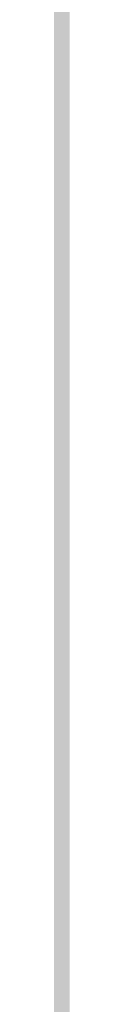
# Model space of a CAD drawing. Units: inches. Extents: x 2083 to 3317, y 1141 to 2115.
# Tile 200 of 256: x 3126.9558 to 3126.9579, y 1263.6134 to 1264.1307. Entities that reach past the tile are written whole.
import ezdxf

# ---------------------------------------------------------------- set-up
doc = ezdxf.new("R2010")
doc.units = ezdxf.units.IN
doc.layers.add('A-ANNO-DIMS', color=2, linetype='Continuous', lineweight=18)
doc.layers.add('A-WALL-PATT', color=251, linetype='Continuous', lineweight=13, true_color=0x636466)
doc.styles.get("Standard").update_dxf_attribs({"font": 'arial.ttf'})
doc.dimstyles.new('ISO-25', dxfattribs={"dimtxt": 12, "dimasz": 12, "dimexe": 1.25, "dimexo": 0.625, "dimtad": 1, "dimlunit": 3, "dimtxsty": 'Standard', "dimcen": 2.5, "dimadec": 0, "dimazin": 0, "dimtfac": 1, "dimtmove": 0, "dimatfit": 3, "dimfxl": 1, "dimarcsym": 0})

# ---------------------------------------------------------------- blocks, each defined once
blk = doc.blocks.new('*D26')
at = {"layer": 'A-ANNO-DIMS', "color": 0, "lineweight": -2, "transparency": 16777216}
for p, q in [((3088.98584, 1274.91509), (3088.98584, 1270.95196)), ((3111.24004, 1274.91509), (3111.24004, 1270.95196)), ((3076.98584, 1272.20196), (2840.26245, 1272.20196)), ((3111.24004, 1272.20196), (3088.98584, 1272.20196)), ((3123.24004, 1272.20196), (3135.24004, 1272.20196))]:
    blk.add_line(p, q, dxfattribs=at)
at = {"layer": 'A-ANNO-DIMS', "color": 0, "transparency": 16777216}
for points in [[(3076.98584, 1274.20196), (3076.98584, 1270.20196), (3088.98584, 1272.20196)], [(3123.24004, 1274.20196), (3123.24004, 1270.20196), (3111.24004, 1272.20196)]]:
    blk.add_solid(points, dxfattribs=at)
at = {"layer": 'Defpoints', "color": 0, "transparency": 16777216}
for p in [(3088.98584, 1275.54009), (3111.24004, 1275.54009), (3088.98584, 1272.20196)]:
    blk.add_point(p, dxfattribs=at)
at = {"layer": 'A-ANNO-DIMS', "color": 0, "transparency": 16777216, "insert": (2952.62415, 1279.0316), "char_height": 12, "attachment_point": 5}
blk.add_mtext('NIGHTSTAND 1\'-10 1/2" TYP.', dxfattribs=at)
blk = doc.blocks.new('*D27')
at = {"layer": 'A-ANNO-DIMS', "color": 0, "lineweight": -2, "transparency": 16777216}
for p, q in [((3114.57817, 1309.79428), (3114.57817, 1321.79428)), ((3111.86504, 1297.79428), (3115.82817, 1297.79428)), ((3114.57817, 1297.79428), (3114.57817, 1275.54009)), ((3111.86504, 1275.54009), (3115.82817, 1275.54009)), ((3114.57817, 1263.54009), (3114.57817, 1140.98859))]:
    blk.add_line(p, q, dxfattribs=at)
at = {"layer": 'A-ANNO-DIMS', "color": 0, "transparency": 16777216}
for points in [[(3112.57817, 1309.79428), (3116.57817, 1309.79428), (3114.57817, 1297.79428)], [(3112.57817, 1263.54009), (3116.57817, 1263.54009), (3114.57817, 1275.54009)]]:
    blk.add_solid(points, dxfattribs=at)
at = {"layer": 'Defpoints', "color": 0, "transparency": 16777216}
for p in [(3111.24004, 1297.79428), (3111.24004, 1275.54009), (3114.57817, 1275.54009)]:
    blk.add_point(p, dxfattribs=at)
at = {"layer": 'A-ANNO-DIMS', "color": 0, "transparency": 16777216, "insert": (3107.74853, 1196.26434), "char_height": 12, "attachment_point": 5, "rotation": 90}
blk.add_mtext('1\'-10 1/2" TYP.', dxfattribs=at)

msp = doc.modelspace()

# ---------------------------------------------------------------- hatches: boundary and pattern name
at = {"layer": 'A-WALL-PATT'}
h = msp.add_hatch(color=256, dxfattribs=at)
h.dxf.hatch_style = 1
h.paths.add_polyline_path([(3126.95978, 2020.76136), (2748.95978, 2020.76136), (2604.95978, 2020.76136), (2226.95978, 2020.76136), (2226.95978, 1702.76136), (2466.95978, 1702.76136), (2466.95978, 1582.76136), (2418.95978, 1582.76136), (2418.95978, 1477.76136), (2226.95978, 1477.76136), (2226.95978, 1263.26136), (2544.95978, 1263.26136), (2544.95978, 1411.76136), (2604.95978, 1411.76136), (2685.95978, 1411.76136), (2685.95978, 1420.76136), (2604.95978, 1420.76136), (2604.95978, 1573.76136), (2604.95978, 1702.76136), (2604.95978, 2011.76136), (2748.95978, 2011.76136), (2748.95978, 1702.76136), (2862.95978, 1702.76136), (2862.95978, 1621.76136), (2871.95978, 1621.76136), (2871.95978, 1702.76136), (2883.95978, 1702.76136), (2883.95978, 1706.93946, -0.026459), (2883.95978, 1711.76136), (2757.95978, 1711.76136), (2757.95978, 1807.76136), (2787.95978, 1807.76136), (2787.95978, 1812.26136), (2757.95978, 1812.26136), (2757.95978, 2011.76136), (2877.95978, 2011.76136), (2877.95978, 1812.26136), (2847.95978, 1812.26136), (2847.95978, 1807.76136), (2889.83574, 1807.76136), (2889.83574, 1812.26136), (2882.45978, 1812.26136), (2882.45978, 2011.76136), (3117.95978, 2011.76136), (3117.95978, 1812.26136), (2937.83574, 1812.26136), (2937.83574, 1807.76136), (2995.70978, 1807.76136), (2995.70978, 1796.11767), (3000.20978, 1796.11767), (3000.20978, 1807.76136), (3117.95978, 1807.76136), (3117.95978, 1711.76136), (3000.20978, 1711.76136), (3000.20978, 1760.11767), (2998.5727, 1760.11767, -0.020711), (2995.70978, 1760.11767), (2995.70978, 1711.76136), (2931.95978, 1711.76136), (2931.95978, 1702.76136), (3126.95978, 1702.76136)])
h.paths.add_polyline_path([(2471.45978, 2011.76136), (2471.45978, 1810.01136), (2462.71694, 1810.01136), (2462.71694, 1805.51136), (2505.95978, 1805.51136), (2505.95978, 1810.01136), (2475.95978, 1810.01136), (2475.95978, 2011.76136), (2595.95978, 2011.76136), (2595.95978, 1810.01136), (2565.95978, 1810.01136), (2565.95978, 1805.51136), (2595.95978, 1805.51136), (2595.95978, 1711.76136), (2235.95978, 1711.76136), (2235.95978, 1805.51136), (2353.70978, 1805.51136), (2353.70978, 1796.05416), (2358.20978, 1796.05416), (2358.20978, 1805.51136), (2414.71694, 1805.51136), (2414.71694, 1810.01136), (2235.95978, 1810.01136), (2235.95978, 2011.76136)], flags=16)
h.paths.add_polyline_path([(2270.20473, 1994.61001), (2270.20473, 1970.61001), (2246.20473, 1970.61001), (2246.20473, 1994.61001)], flags=0)
edge = h.paths.add_edge_path(flags=0)
edge.add_ellipse((2332.02739, 1899.79818), major_axis=(-3.04299, 3.04299), ratio=0.1682525, start_angle=-161.33217, end_angle=-156.30711, ccw=False)
edge.add_ellipse((2333.08204, 1898.74353), major_axis=(-1.05465, 1.05465), ratio=0.4535321, start_angle=-123.37102, end_angle=-94.15911)
edge = h.paths.add_edge_path(flags=0)
edge.add_ellipse((2332.02739, 1968.87629), major_axis=(3.04299, 3.04299), ratio=0.1682525, start_angle=18.66783, end_angle=23.69289)
edge.add_spline(control_points=[(2332.9256, 1970.6911), (2332.22677, 1970.3361), (2330.89371, 1969.65891), (2328.41308, 1970.93214), (2327.20393, 1967.74871), (2324.7096, 1969.95559), (2322.53282, 1967.01235), (2320.01285, 1971.29581), (2317.68031, 1968.15784), (2316.04053, 1967.10205), (2315.4269, 1966.8096)], knot_values=[0, 0, 0, 0, 2.267059, 4.324559, 6.685584, 8.878641, 11.121502, 14.300359, 17.755284, 19.732645, 19.732645, 19.732645, 19.732645], degree=3, periodic=0)
edge.add_ellipse((2332.02739, 1968.87629), major_axis=(3.04299, 3.04299), ratio=0.1682525, start_angle=18.66783, end_angle=23.69289, ccw=False)
edge.add_ellipse((2333.08204, 1969.93094), major_axis=(1.05465, 1.05465), ratio=0.4535321, start_angle=56.62898, end_angle=85.84089, ccw=False)
edge = h.paths.add_edge_path(flags=0)
edge.add_spline(control_points=[(2296.42829, 1967.98791), (2293.6278, 1965.33631), (2287.70362, 1959.72709), (2299.74386, 1949.9957), (2294.53259, 1935.66853), (2290.57323, 1920.60351), (2293.39412, 1909.97369), (2296.18541, 1904.96654)], knot_values=[0.099185, 0.099185, 0.099185, 0.099185, 0.345301, 0.619822, 0.982653, 1.386093, 1.810555, 1.810555, 1.810555, 1.810555], degree=3, periodic=0)
edge.add_spline(control_points=[(2296.18541, 1904.96654), (2297.38358, 1902.6193), (2298.00097, 1901.94931), (2298.55297, 1901.46815)], knot_values=[0.006246, 0.006246, 0.006246, 0.006246, 0.055476, 0.055476, 0.055476, 0.055476], degree=3, periodic=0)
edge.add_spline(control_points=[(2298.55297, 1901.46815), (2297.25861, 1900.92322), (2295.22529, 1900.23213), (2293.06023, 1900.61421), (2292.10142, 1900.78841), (2292.08958, 1900.79057)], knot_values=[0.312835, 0.312835, 0.312835, 0.312835, 0.40178, 0.474987, 0.475903, 0.475903, 0.475903, 0.475903], degree=3, periodic=0)
edge.add_arc((2292.79365, 1904.66411), 3.93701, 215.4209, 259.69818, ccw=False)
edge.add_spline(control_points=[(2289.58531, 1902.3823), (2289.47665, 1902.53509), (2289.36848, 1902.68804), (2289.26086, 1902.84117)], knot_values=[0.102872, 0.102872, 0.102872, 0.102872, 0.116896, 0.116896, 0.116896, 0.116896], degree=3, periodic=0)
edge.add_spline(control_points=[(2289.26086, 1902.84117), (2288.6866, 1902.55019), (2287.64005, 1902.0199), (2285.88134, 1901.87395), (2283.85297, 1901.50435), (2281.71999, 1899.71054), (2278.46699, 1899.49294), (2276.15714, 1901.8832), (2272.25895, 1899.80407), (2267.77761, 1901.84318), (2262.24388, 1900.18403), (2257.41493, 1901.78206), (2254.31837, 1900.72612), (2253.17828, 1900.33734)], knot_values=[0, 0, 0, 0, 1.907977, 3.477176, 5.261074, 7.972851, 11.680248, 13.717921, 16.939592, 22.789562, 27.502503, 33.595215, 37.145618, 37.145618, 37.145618, 37.145618], degree=3, periodic=0)
edge.add_line((2253.17828, 1900.33734), (2250.24424, 1902.84117))
edge.add_line((2250.24424, 1902.84117), (2250.24424, 1965.8333))
edge.add_line((2250.24424, 1965.8333), (2253.17828, 1968.33712))
edge.add_spline(control_points=[(2253.17828, 1968.33712), (2254.31837, 1967.94835), (2257.41493, 1966.89241), (2262.24388, 1968.49043), (2267.77761, 1966.83128), (2271.52673, 1968.53722), (2273.87591, 1967.82829), (2274.2067, 1967.72764)], knot_values=[0, 0, 0, 0, 0.09018, 0.244935, 0.364644, 0.513233, 0.537855, 0.537855, 0.537855, 0.537855], degree=3, periodic=0)
edge.add_arc((2274.35289, 1963.79335), 3.93701, 72.05113, 92.12795, ccw=False)
edge.add_arc((2281.29693, 1985.23), 18.5963, 252.051134, 288.565722)
edge.add_arc((2292.31672, 1956.02888), 12.64608, 71.026788, 113.778218, ccw=False)
edge = h.paths.add_edge_path(flags=0)
edge.add_spline(control_points=[(2274.89941, 1951.85619), (2275.06616, 1951.61659), (2275.23269, 1951.37659), (2275.39799, 1951.13585)], knot_values=[1.409916, 1.409916, 1.409916, 1.409916, 1.43159, 1.43159, 1.43159, 1.43159], degree=3, periodic=0)
edge.add_spline(control_points=[(2275.39799, 1951.13585), (2275.79211, 1950.56189), (2276.17923, 1949.98377), (2276.54555, 1949.3971)], knot_values=[1.358238, 1.358238, 1.358238, 1.358238, 1.409916, 1.409916, 1.409916, 1.409916], degree=3, periodic=0)
edge.add_line((2276.54555, 1949.3971), (2277.43729, 1947.86218))
edge.add_spline(control_points=[(2277.43729, 1947.86218), (2276.30383, 1945.67311), (2274.6397, 1942.42688), (2274.63161, 1938.0939), (2272.79912, 1930.85155), (2274.35643, 1943.89705), (2275.94768, 1947.92336), (2276.54555, 1949.3971)], knot_values=[0.005632, 0.005632, 0.005632, 0.005632, 0.186014, 0.266002, 0.357087, 0.59639, 0.739732, 0.739732, 0.739732, 0.739732], degree=3, periodic=0)
edge.add_spline(control_points=[(2276.54555, 1949.3971), (2276.17923, 1949.98377), (2275.79211, 1950.56189), (2275.39799, 1951.13585)], knot_values=[1.358238, 1.358238, 1.358238, 1.358238, 1.409916, 1.409916, 1.409916, 1.409916], degree=3, periodic=0)
edge.add_spline(control_points=[(2275.39799, 1951.13585), (2274.9425, 1950.08045), (2274.20776, 1948.02527), (2273.9346, 1944.85148), (2272.46853, 1937.62749), (2273.46622, 1945.69647), (2274.70062, 1951.05947), (2274.89941, 1951.85619)], knot_values=[0.104364, 0.104364, 0.104364, 0.104364, 0.189636, 0.269624, 0.36071, 0.600013, 0.644622, 0.644622, 0.644622, 0.644622], degree=3, periodic=0)
h.paths.add_polyline_path([(2269.16751, 1963.12757, -0.357527), (2268.17063, 1960.97637, -0.092561), (2268.17063, 1939.43632, -0.357527), (2269.16751, 1937.28512, -0.357527), (2267.01631, 1938.282, -0.164785), (2254.68558, 1938.282, -0.357527), (2252.53438, 1937.28512, -0.357527), (2253.53126, 1939.43632, -0.092561), (2253.53126, 1960.97637, -0.357527), (2252.53438, 1963.12757, -0.357527), (2254.68558, 1962.13069, -0.164785), (2267.01631, 1962.13069, -0.357527)], flags=0)
h.paths.add_polyline_path([(2248.87407, 1967.8018), (2248.87407, 1957.02771), (2249.45778, 1957.02771), (2249.45778, 1911.64676), (2248.87407, 1911.64676), (2248.87407, 1900.87267), (2246.51186, 1900.87267, 0.197327), (2244.14966, 1902.45687), (2244.14966, 1966.21759, 0.197327), (2246.51186, 1967.8018)], flags=0)
h.paths.add_polyline_path([(2269.16751, 1931.38934, -0.357527), (2268.17063, 1929.23814, -0.092561), (2268.17063, 1907.6981, -0.357527), (2269.16751, 1905.54689, -0.357527), (2267.01631, 1906.54377, -0.164785), (2254.68558, 1906.54377, -0.357527), (2252.53438, 1905.54689, -0.357527), (2253.53126, 1907.6981, -0.092561), (2253.53126, 1929.23814, -0.357527), (2252.53438, 1931.38934, -0.357527), (2254.68558, 1930.39246, -0.164785), (2267.01631, 1930.39246, -0.357527)], flags=0)
edge = h.paths.add_edge_path(flags=0)
edge.add_spline(control_points=[(2276.19686, 1906.7237), (2276.16814, 1909.02893), (2276.11405, 1913.37185), (2270.59842, 1924.92498), (2273.90517, 1919.01278), (2275.92171, 1916.26206), (2275.47457, 1912.40215), (2277.25787, 1910.38062), (2276.69604, 1908.22504), (2276.64622, 1906.81302), (2276.61782, 1906.00841)], knot_values=[0, 0, 0, 0, 8.61026, 16.221274, 18.843057, 23.804898, 27.440828, 29.356102, 31.203478, 33.650687, 33.650687, 33.650687, 33.650687], degree=3, periodic=0)
edge.add_spline(control_points=[(2276.61782, 1906.00841), (2276.62331, 1905.62414), (2276.49774, 1904.62866), (2275.44178, 1903.85473), (2274.93731, 1903.08045), (2274.85908, 1902.84117)], knot_values=[0.156488, 0.156488, 0.156488, 0.156488, 0.184398, 0.231376, 0.250598, 0.250598, 0.250598, 0.250598], degree=3, periodic=0)
edge.add_line((2274.85908, 1902.84117), (2276.50598, 1902.84117))
edge.add_spline(control_points=[(2276.50598, 1902.84117), (2276.78831, 1903.08494), (2277.66507, 1904.1252), (2278.24954, 1904.34074), (2277.65387, 1908.52739), (2278.15567, 1906.22781), (2278.10046, 1905.28595), (2278.84667, 1904.06901), (2277.85679, 1903.41495), (2277.87419, 1902.99105), (2277.90356, 1902.84117)], knot_values=[0.059574, 0.059574, 0.059574, 0.059574, 0.080753, 0.103741, 0.16972, 0.176036, 0.207137, 0.240474, 0.262341, 0.27366, 0.27366, 0.27366, 0.27366], degree=3, periodic=0)
edge.add_line((2277.90356, 1902.84117), (2280.02983, 1902.84117))
edge.add_spline(control_points=[(2280.02983, 1902.84117), (2279.88822, 1903.0884), (2279.49926, 1903.98155), (2280.15228, 1905.93935), (2278.10362, 1909.65776), (2279.76239, 1907.18529), (2280.3279, 1904.87486), (2280.48511, 1903.48959), (2281.46327, 1903.24943), (2281.75834, 1902.9365), (2281.83404, 1902.84117)], knot_values=[0.013856, 0.013856, 0.013856, 0.013856, 0.034874, 0.088867, 0.107879, 0.126738, 0.158714, 0.193757, 0.217487, 0.226722, 0.226722, 0.226722, 0.226722], degree=3, periodic=0)
edge.add_spline(control_points=[(2281.83404, 1902.84117), (2281.78753, 1902.8267), (2281.64702, 1902.78299), (2281.39553, 1902.85949), (2281.08808, 1902.98524), (2280.72068, 1903.0609), (2280.33345, 1903.02573), (2280.12477, 1902.89888), (2280.02983, 1902.84117)], knot_values=[0, 0, 0, 0, 0.14413, 0.435517, 0.749276, 1.153046, 1.548371, 1.878348, 1.878348, 1.878348, 1.878348], degree=3, periodic=0)
edge.add_line((2280.02983, 1902.84117), (2277.90356, 1902.84117))
edge.add_spline(control_points=[(2277.90356, 1902.84117), (2277.89286, 1902.79586), (2277.8654, 1902.67964), (2277.60748, 1902.68748), (2277.27405, 1902.8007), (2276.83792, 1902.61977), (2276.58381, 1902.78926), (2276.50598, 1902.84117)], knot_values=[0, 0, 0, 0, 0.127189, 0.326199, 0.628009, 1.24357, 1.515331, 1.515331, 1.515331, 1.515331], degree=3, periodic=0)
edge.add_line((2276.50598, 1902.84117), (2274.85908, 1902.84117))
edge.add_spline(control_points=[(2274.85908, 1902.84117), (2274.81444, 1902.89859), (2274.72513, 1903.01345), (2274.49348, 1903.11897), (2274.24429, 1902.96054), (2273.93712, 1903.18494), (2273.61404, 1902.98314), (2273.40832, 1902.88304), (2273.32225, 1902.84117)], knot_values=[0, 0, 0, 0, 0.21843, 0.436957, 0.687977, 0.990379, 1.398396, 1.69185, 1.69185, 1.69185, 1.69185], degree=3, periodic=0)
edge.add_spline(control_points=[(2273.32225, 1902.84117), (2273.61674, 1903.44569), (2274.274, 1904.53825), (2276.02724, 1904.5737), (2276.20696, 1906.58364), (2276.19686, 1906.7237)], knot_values=[0.012227, 0.012227, 0.012227, 0.012227, 0.059472, 0.106218, 0.134458, 0.134458, 0.134458, 0.134458], degree=3, periodic=0)
h.paths.add_polyline_path([(2270.77605, 1897.78983), (2270.77605, 1873.78983), (2246.77605, 1873.78983), (2246.77605, 1897.78983)], flags=0)
h.paths.add_polyline_path([(2353.70978, 1760.00506), (2353.70978, 1760.05416), (2358.20978, 1760.05416, -0.033729)], flags=0)
h.paths.add_polyline_path([(2321.81912, 1737.52919), (2341.99533, 1737.52919, -0.414214), (2343.20327, 1736.32124), (2343.20327, 1721.0206, -0.414214), (2341.99533, 1719.81265), (2321.81912, 1719.81265, -0.414214), (2320.61117, 1721.0206), (2320.61117, 1736.32124, -0.414214)], flags=0)
h.paths.add_polyline_path([(2324.23501, 1736.32124), (2339.57944, 1736.32124, -0.414214), (2341.99533, 1733.90535), (2341.99533, 1725.44973, -0.414214), (2339.57944, 1723.03384), (2333.68059, 1723.03384), (2333.84532, 1722.04547, -0.870646), (2335.4254, 1721.82589, -0.767327), (2333.92269, 1721.42324), (2331.29102, 1721.42324, -0.767327), (2329.78832, 1721.82589, -0.870646), (2331.3684, 1722.04547), (2331.53313, 1723.03384), (2324.23501, 1723.03384, -0.414214), (2321.81912, 1725.44973), (2321.81912, 1733.90535, -0.414214)], flags=0)
h.paths.add_polyline_path([(2570.48379, 1928.61544), (2589.68379, 1928.61544), (2590.16883, 1928.61544), (2590.16883, 1904.9934), (2570.48379, 1904.9934)], flags=0)
h.paths.add_polyline_path([(2574.44732, 1927.26382, -1), (2572.82884, 1927.26382, -1)], flags=0)
h.paths.add_polyline_path([(2573.08987, 1926.94088), (2573.92503, 1927.77604), (2574.14774, 1927.55333), (2573.31258, 1926.71817)], flags=0)
h.paths.add_polyline_path([(2578.77906, 1919.72962, -1), (2571.59166, 1919.72962, -1)], flags=0)
h.paths.add_polyline_path([(2578.38536, 1919.72962, -1), (2571.98536, 1919.72962, -1)], flags=0)
h.paths.add_polyline_path([(2331.59576, 1729.47622, -1), (2333.61795, 1729.47622, -1)], flags=0)
h.paths.add_polyline_path([(2578.03423, 1927.26382, -1), (2576.41574, 1927.26382, -1)], flags=0)
h.paths.add_polyline_path([(2576.68885, 1927.53109), (2576.91156, 1927.7538), (2577.74673, 1926.91863), (2577.52402, 1926.69592)], flags=0)
h.paths.add_polyline_path([(2578.13906, 1909.85954, -1), (2572.23166, 1909.85954, -1)], flags=0)
h.paths.add_polyline_path([(2577.74536, 1909.85954, -1), (2572.62536, 1909.85954, -1)], flags=0)
h.paths.add_polyline_path([(2583.79772, 1927.26382, -1), (2582.17923, 1927.26382, -1)], flags=0)
h.paths.add_polyline_path([(2582.71865, 1927.7538), (2583.55381, 1926.91863), (2583.3311, 1926.69592), (2582.49594, 1927.53109)], flags=0)
h.paths.add_polyline_path([(2582.49594, 1927.53109), (2582.71865, 1927.7538), (2583.55381, 1926.91863), (2583.3311, 1926.69592)], flags=0)
h.paths.add_polyline_path([(2587.73906, 1920.52962, -1), (2581.83166, 1920.52962, -1)], flags=0)
h.paths.add_polyline_path([(2587.34536, 1920.52962, -1), (2582.22536, 1920.52962, -1)], flags=0)
h.paths.add_polyline_path([(2587.38462, 1927.26382, -1), (2585.76613, 1927.26382, -1)], flags=0)
h.paths.add_polyline_path([(2586.08199, 1926.98025), (2586.91716, 1927.81541), (2587.13987, 1927.5927), (2586.3047, 1926.75754)], flags=0)
h.paths.add_polyline_path([(2588.37906, 1910.65954, -1), (2581.19166, 1910.65954, -1)], flags=0)
h.paths.add_polyline_path([(2587.98536, 1910.65954, -1), (2581.58536, 1910.65954, -1)], flags=0)
h.paths.add_polyline_path([(2417.16773, 1729.4779), (2437.34394, 1729.4779, -0.414214), (2438.55188, 1728.26995), (2438.55188, 1712.96931, -0.414214), (2437.34394, 1711.76136), (2417.16773, 1711.76136, -0.414214), (2415.95978, 1712.96931), (2415.95978, 1728.26995, -0.414214)], flags=0)
h.paths.add_polyline_path([(2419.58362, 1728.26995), (2434.92805, 1728.26995, -0.414214), (2437.34394, 1725.85406), (2437.34394, 1717.39844, -0.414214), (2434.92805, 1714.98255), (2429.0292, 1714.98255), (2429.19393, 1713.99418, -0.870646), (2430.77401, 1713.7746, -0.767327), (2429.2713, 1713.37195), (2426.63963, 1713.37195, -0.767327), (2425.13693, 1713.7746, -0.870646), (2426.71701, 1713.99418), (2426.88174, 1714.98255), (2419.58362, 1714.98255, -0.414214), (2417.16773, 1717.39844), (2417.16773, 1725.85406, -0.414214)], flags=0)
h.paths.add_polyline_path([(2419.58362, 1728.26995), (2434.92805, 1728.26995, -0.414214), (2437.34394, 1725.85406), (2437.34394, 1717.39844, -0.414214), (2434.92805, 1714.98255), (2429.0292, 1714.98255), (2428.35812, 1719.00903), (2427.55282, 1719.00903), (2426.88174, 1714.98255), (2419.58362, 1714.98255, -0.414214), (2417.16773, 1717.39844), (2417.16773, 1725.85406, -0.414214)], flags=0)
h.paths.add_polyline_path([(2426.94437, 1721.42492, -1), (2428.96656, 1721.42492, -1)], flags=0)
h.paths.add_polyline_path([(2475.95978, 1702.76136), (2595.95978, 1702.76136), (2595.95978, 1582.76136), (2475.95978, 1582.76136)], flags=16)
h.paths.add_polyline_path([(2427.95978, 1573.76136), (2595.95978, 1573.76136), (2595.95978, 1468.76136), (2595.95978, 1420.76136), (2384.45978, 1420.76136), (2384.45978, 1468.76136), (2427.95978, 1468.76136)], flags=16)
h.paths.add_polyline_path([(2379.95978, 1468.76136), (2379.95978, 1420.76136), (2235.95978, 1420.76136), (2235.95978, 1468.76136)], flags=16)
h.paths.add_polyline_path([(2317.816, 1466.69577), (2337.9922, 1466.69577, -0.414214), (2339.20015, 1465.48782), (2339.20015, 1450.18718, -0.414214), (2337.9922, 1448.97923), (2317.816, 1448.97923, -0.414214), (2316.60805, 1450.18718), (2316.60805, 1465.48782, -0.414214)], flags=0)
h.paths.add_polyline_path([(2320.23189, 1465.48782), (2335.57631, 1465.48782, -0.414214), (2337.9922, 1463.07193), (2337.9922, 1454.61631, -0.414214), (2335.57631, 1452.20042), (2329.67747, 1452.20042), (2329.84219, 1451.21205, -0.870646), (2331.42228, 1450.99247, -0.767327), (2329.91957, 1450.58983), (2327.2879, 1450.58983, -0.767327), (2325.7852, 1450.99247, -0.870646), (2327.36528, 1451.21205), (2327.53001, 1452.20042), (2320.23189, 1452.20042, -0.414214), (2317.816, 1454.61631), (2317.816, 1463.07193, -0.414214)], flags=0)
h.paths.add_polyline_path([(2320.23189, 1465.48782), (2335.57631, 1465.48782, -0.414214), (2337.9922, 1463.07193), (2337.9922, 1454.61631, -0.414214), (2335.57631, 1452.20042), (2329.67747, 1452.20042), (2329.00638, 1456.22691), (2328.20109, 1456.22691), (2327.53001, 1452.20042), (2320.23189, 1452.20042, -0.414214), (2317.816, 1454.61631), (2317.816, 1463.07193, -0.414214)], flags=0)
h.paths.add_polyline_path([(2327.59264, 1458.6428, -1), (2329.61483, 1458.6428, -1)], flags=0)
h.paths.add_polyline_path([(2244.41174, 1433.34045), (2241.92094, 1433.34045, -0.414214), (2240.01786, 1435.24354), (2240.01786, 1440.95281, -0.414211), (2241.92093, 1442.8559), (2244.41174, 1442.8559, -1.976472)], flags=0)
h.paths.add_polyline_path([(2245.35689, 1434.39754, -0.414214), (2245.35689, 1441.79881, -2.144098)], flags=0)
h.paths.add_polyline_path([(2535.95978, 1416.26136), (2535.95978, 1272.26136), (2235.95978, 1272.26136), (2235.95978, 1416.26136)], flags=16)
h.paths.add_polyline_path([(2260.11956, 1384.29284), (2260.11956, 1362.03865), (2237.86537, 1362.03865), (2237.86537, 1384.29284)], flags=0)
edge = h.paths.add_edge_path(flags=0)
edge.add_line((2318.25185, 1362.0933), (2318.1458, 1362.00097))
edge.add_ellipse((2317.44512, 1360.43104), major_axis=(2.82164, 2.82164), ratio=0.1682525, start_angle=18.66783, end_angle=20.94813, ccw=False)
edge.add_ellipse((2318.42305, 1361.40897), major_axis=(0.97793, 0.97793), ratio=0.4535321, start_angle=56.62898, end_angle=70.2262, ccw=False)
edge = h.paths.add_edge_path(flags=0)
edge.add_line((2319.10737, 1295.57108), (2319.01504, 1295.67713))
edge.add_ellipse((2317.44512, 1296.37781), major_axis=(-2.82164, 2.82164), ratio=0.1682525, start_angle=-161.33217, end_angle=-159.05187, ccw=False)
edge.add_ellipse((2318.42305, 1295.39988), major_axis=(-0.97793, 0.97793), ratio=0.4535321, start_angle=-123.37102, end_angle=-109.7738)
edge = h.paths.add_edge_path(flags=0)
edge.add_spline(control_points=[(2284.21035, 1301.17022), (2284.58069, 1300.44472), (2284.89119, 1299.89202), (2285.15955, 1299.46102)], knot_values=[0.039066, 0.039066, 0.039066, 0.039066, 0.055476, 0.055476, 0.055476, 0.055476], degree=3, periodic=0)
edge.add_line((2285.15955, 1299.46102), (2284.21035, 1301.17022))
edge = h.paths.add_edge_path(flags=0)
edge.add_line((2280.41246, 1297.29801), (2283.36999, 1297.03612))
edge.add_line((2283.36999, 1297.03612), (2286.40569, 1297.92631))
edge.add_spline(control_points=[(2286.40569, 1297.92631), (2285.30549, 1297.46312), (2284.34478, 1297.12915), (2283.36999, 1297.03612)], knot_values=[0.394369, 0.394369, 0.394369, 0.394369, 0.475903, 0.475903, 0.475903, 0.475903], degree=3, periodic=0)
edge.add_spline(control_points=[(2283.36999, 1297.03612), (2283.28139, 1297.02767), (2282.31629, 1296.95734), (2281.3125, 1297.13448), (2280.42344, 1297.29602), (2280.41246, 1297.29801)], knot_values=[0.312835, 0.312835, 0.312835, 0.312835, 0.320246, 0.393453, 0.394369, 0.394369, 0.394369, 0.394369], degree=3, periodic=0)
edge = h.paths.add_edge_path(flags=0)
edge.add_line((2284.43556, 1359.60729), (2280.44629, 1355.32805))
edge.add_line((2280.44629, 1355.32805), (2279.57999, 1351.01775))
edge.add_line((2279.57999, 1351.01775), (2282.41297, 1346.58043))
edge.add_spline(control_points=[(2282.41297, 1346.58043), (2283.15333, 1345.58924), (2284.2529, 1344.0289), (2284.80104, 1342.38717), (2284.93516, 1341.80554)], knot_values=[1.240098, 1.240098, 1.240098, 1.240098, 1.332892, 1.382712, 1.382712, 1.382712, 1.382712], degree=3, periodic=0)
edge.add_spline(control_points=[(2284.93516, 1341.80554), (2285.31911, 1340.1406), (2285.23303, 1338.4092), (2284.90994, 1336.65412)], knot_values=[1.097484, 1.097484, 1.097484, 1.097484, 1.240098, 1.240098, 1.240098, 1.240098], degree=3, periodic=0)
edge.add_spline(control_points=[(2284.90994, 1336.65412), (2284.58685, 1334.89904), (2284.02675, 1333.12027), (2283.46264, 1331.36058)], knot_values=[0.95487, 0.95487, 0.95487, 0.95487, 1.097484, 1.097484, 1.097484, 1.097484], degree=3, periodic=0)
edge.add_line((2283.46264, 1331.36058), (2281.89038, 1326.15336))
edge.add_line((2281.89038, 1326.15336), (2280.75626, 1321.05609))
edge.add_line((2280.75626, 1321.05609), (2280.2992, 1316.00198))
edge.add_line((2280.2992, 1316.00198), (2280.71593, 1310.95007))
edge.add_line((2280.71593, 1310.95007), (2282.02809, 1305.97214))
edge.add_line((2282.02809, 1305.97214), (2284.21035, 1301.17022))
edge.add_spline(control_points=[(2284.21035, 1301.17022), (2283.34073, 1302.73019), (2282.6119, 1304.33649), (2282.02809, 1305.97214)], knot_values=[0.099185, 0.099185, 0.099185, 0.099185, 0.241799, 0.241799, 0.241799, 0.241799], degree=3, periodic=0)
edge.add_spline(control_points=[(2282.02809, 1305.97214), (2281.44428, 1307.60778), (2281.00549, 1309.27276), (2280.71593, 1310.95007)], knot_values=[0.241799, 0.241799, 0.241799, 0.241799, 0.384413, 0.384413, 0.384413, 0.384413], degree=3, periodic=0)
edge.add_spline(control_points=[(2280.71593, 1310.95007), (2280.43324, 1312.58761), (2280.28939, 1314.27696), (2280.29889, 1315.96203), (2280.2992, 1316.00198)], knot_values=[0.384413, 0.384413, 0.384413, 0.384413, 0.523647, 0.527028, 0.527028, 0.527028, 0.527028], degree=3, periodic=0)
edge.add_spline(control_points=[(2280.2992, 1316.00198), (2280.31233, 1317.68696), (2280.47787, 1319.36793), (2280.75626, 1321.05609)], knot_values=[0.527028, 0.527028, 0.527028, 0.527028, 0.669642, 0.669642, 0.669642, 0.669642], degree=3, periodic=0)
edge.add_spline(control_points=[(2280.75626, 1321.05609), (2281.03465, 1322.74425), (2281.42588, 1324.43961), (2281.89038, 1326.15336)], knot_values=[0.669642, 0.669642, 0.669642, 0.669642, 0.812256, 0.812256, 0.812256, 0.812256], degree=3, periodic=0)
edge.add_spline(control_points=[(2281.89038, 1326.15336), (2282.26438, 1327.53325), (2282.78787, 1329.26181), (2283.35275, 1331.01778), (2283.46264, 1331.36058)], knot_values=[0.812256, 0.812256, 0.812256, 0.812256, 0.927087, 0.95487, 0.95487, 0.95487, 0.95487], degree=3, periodic=0)
edge.add_line((2283.46264, 1331.36058), (2284.90994, 1336.65412))
edge.add_line((2284.90994, 1336.65412), (2284.93516, 1341.80554))
edge.add_line((2284.93516, 1341.80554), (2282.41297, 1346.58043))
edge.add_spline(control_points=[(2282.41297, 1346.58043), (2281.27513, 1348.10379), (2280.07845, 1349.57032), (2279.57999, 1351.01775)], knot_values=[1.382712, 1.382712, 1.382712, 1.382712, 1.525326, 1.525326, 1.525326, 1.525326], degree=3, periodic=0)
edge.add_spline(control_points=[(2279.57999, 1351.01775), (2279.44328, 1351.41472), (2279.13631, 1352.85692), (2279.73519, 1354.29039), (2280.44629, 1355.32805)], knot_values=[1.525326, 1.525326, 1.525326, 1.525326, 1.564439, 1.667941, 1.667941, 1.667941, 1.667941], degree=3, periodic=0)
edge.add_spline(control_points=[(2280.44629, 1355.32805), (2281.42611, 1356.75784), (2282.93084, 1358.18256), (2284.43556, 1359.60729)], knot_values=[1.667941, 1.667941, 1.667941, 1.667941, 1.810555, 1.810555, 1.810555, 1.810555], degree=3, periodic=0)
edge.add_arc((2280.62307, 1348.51818), 11.72618, 71.026788, 113.778218)
edge.add_arc((2270.40489, 1375.59516), 17.24357, 252.051134, 288.565722, ccw=False)
edge.add_arc((2263.96597, 1355.71785), 3.65062, 72.05113, 92.12795)
edge.add_arc((2263.96597, 1355.71785), 3.65062, 92.12795, 177.98513)
edge.add_spline(control_points=[(2260.3176, 1355.8462), (2260.26042, 1354.22067), (2260.55128, 1350.18655), (2262.99934, 1346.76625), (2264.47274, 1344.64902)], knot_values=[1.43159, 1.43159, 1.43159, 1.43159, 1.564144, 1.770695, 1.770695, 1.770695, 1.770695], degree=3, periodic=0)
edge.add_line((2264.47274, 1344.64902), (2264.93559, 1343.98253))
edge.add_spline(control_points=[(2263.80104, 1340.24811), (2263.84324, 1340.51409), (2264.06724, 1341.75647), (2264.51269, 1343.00245), (2264.93505, 1343.98108)], knot_values=[0.53657, 0.53657, 0.53657, 0.53657, 0.559349, 0.644622, 0.644622, 0.644622, 0.644622], degree=3, periodic=0)
edge.add_spline(control_points=[(2264.93505, 1343.98108), (2265.11777, 1343.71497), (2265.29888, 1343.44791), (2265.47676, 1343.17936)], knot_values=[1.384077, 1.384077, 1.384077, 1.384077, 1.409916, 1.409916, 1.409916, 1.409916], degree=3, periodic=0)
edge.add_spline(control_points=[(2265.47676, 1343.17936), (2265.65464, 1342.91082), (2265.8293, 1342.64081), (2265.99913, 1342.36881)], knot_values=[1.358238, 1.358238, 1.358238, 1.358238, 1.384077, 1.384077, 1.384077, 1.384077], degree=3, periodic=0)
edge.add_line((2265.99913, 1342.36881), (2266.82601, 1340.94555))
edge.add_spline(control_points=[(2266.82601, 1340.94555), (2268.8944, 1337.08969), (2271.39817, 1325.843), (2270.51616, 1310.56856), (2275.91938, 1301.86061), (2277.78951, 1299.19945)], knot_values=[0.116896, 0.116896, 0.116896, 0.116896, 0.472987, 1.050969, 1.313793, 1.313793, 1.313793, 1.313793], degree=3, periodic=0)
edge.add_spline(control_points=[(2277.78951, 1299.19945), (2277.83941, 1299.12845), (2277.88943, 1299.0575), (2277.93957, 1298.98658)], knot_values=[0.109884, 0.109884, 0.109884, 0.109884, 0.116896, 0.116896, 0.116896, 0.116896], degree=3, periodic=0)
edge.add_line((2277.93957, 1298.98658), (2277.78885, 1299.19911))
edge.add_spline(control_points=[(2277.78885, 1299.19911), (2277.25658, 1298.92941), (2276.28635, 1298.4379), (2275.03935, 1298.33442), (2274.38333, 1298.2389), (2274.21525, 1298.20934)], knot_values=[33.12187, 33.12187, 33.12187, 33.12187, 35.029056, 36.598255, 37.144827, 37.144827, 37.144827, 37.144827], degree=3, periodic=0)
edge.add_line((2274.21525, 1298.20934), (2273.07315, 1297.89296))
edge.add_spline(control_points=[(2273.07315, 1297.89296), (2272.32294, 1297.57978), (2271.03915, 1296.51051), (2269.24839, 1296.22606), (2268.4231, 1296.37465)], knot_values=[26.532584, 26.532584, 26.532584, 26.532584, 29.198919, 31.839101, 31.839101, 31.839101, 31.839101], degree=3, periodic=0)
edge.add_line((2268.4231, 1296.37465), (2263.8785, 1297.45753))
edge.add_spline(control_points=[(2263.8785, 1297.45753), (2263.55608, 1297.35943), (2261.86031, 1296.83869), (2260.23878, 1297.28241), (2258.93345, 1297.51646)], knot_values=[15.919551, 15.919551, 15.919551, 15.919551, 16.939592, 21.226067, 21.226067, 21.226067, 21.226067], degree=3, periodic=0)
edge.add_line((2258.93345, 1297.51646), (2254.05523, 1297.32901))
edge.add_spline(control_points=[(2254.05523, 1297.32901), (2253.75553, 1297.29582), (2252.11368, 1297.16517), (2250.46187, 1297.54422), (2249.12969, 1297.66788)], knot_values=[5.306517, 5.306517, 5.306517, 5.306517, 6.276435, 10.613034, 10.613034, 10.613034, 10.613034], degree=3, periodic=0)
edge.add_line((2249.12969, 1297.66788), (2244.33165, 1296.87776))
edge.add_line((2244.33165, 1296.87776), (2241.61103, 1299.19945))
edge.add_line((2241.61103, 1299.19945), (2241.61103, 1357.6094))
edge.add_line((2241.61103, 1357.6094), (2244.33165, 1359.9311))
edge.add_line((2244.33165, 1359.9311), (2252.72882, 1359.54269))
edge.add_spline(control_points=[(2252.72882, 1359.54269), (2252.87094, 1359.54644), (2253.30574, 1359.54817), (2253.73984, 1359.51427), (2254.03174, 1359.48243)], knot_values=[0.233291, 0.233291, 0.233291, 0.233291, 0.244935, 0.268927, 0.268927, 0.268927, 0.268927], degree=3, periodic=0)
edge.add_line((2254.03174, 1359.48243), (2259.58719, 1359.41639))
edge.add_spline(control_points=[(2259.58719, 1359.41639), (2260.67707, 1359.6285), (2262.0732, 1359.897), (2263.52369, 1359.45928), (2263.83042, 1359.36595)], knot_values=[0.422516, 0.422516, 0.422516, 0.422516, 0.513233, 0.537855, 0.537855, 0.537855, 0.537855], degree=3, periodic=0)
edge.add_arc((2263.96597, 1355.71785), 3.65062, 72.05113, 92.12795, ccw=False)
edge.add_arc((2270.40489, 1375.59516), 17.24357, 252.051134, 288.565722)
edge.add_arc((2280.62307, 1348.51818), 11.72618, 71.026788, 113.778218, ccw=False)
h.paths.add_polyline_path([(2240.34053, 1359.43471), (2240.34053, 1349.44435), (2240.88178, 1349.44435), (2240.88178, 1307.3645), (2240.34053, 1307.3645), (2240.34053, 1297.37414), (2238.15016, 1297.37414, 0.197327), (2235.95978, 1298.84311), (2235.95978, 1357.96575, 0.197327), (2238.15016, 1359.43471)], flags=0)
h.paths.add_polyline_path([(2259.15779, 1355.1005, -0.357527), (2258.23342, 1353.10578, -0.092561), (2258.23342, 1333.1326, -0.357527), (2259.15779, 1331.13788, -0.357527), (2257.16307, 1332.06225, -0.164785), (2245.7293, 1332.06225, -0.357527), (2243.73458, 1331.13788, -0.357527), (2244.65895, 1333.1326, -0.092561), (2244.65895, 1353.10578, -0.357527), (2243.73458, 1355.1005, -0.357527), (2245.7293, 1354.17613, -0.164785), (2257.16307, 1354.17613, -0.357527)], flags=0)
edge = h.paths.add_edge_path(flags=0)
edge.add_line((2265.99913, 1342.36881), (2266.82601, 1340.94555))
edge.add_line((2266.82601, 1340.94555), (2265.30756, 1337.81407))
edge.add_line((2265.30756, 1337.81407), (2264.35823, 1334.65294))
edge.add_line((2264.35823, 1334.65294), (2264.26201, 1333.7997))
edge.add_spline(control_points=[(2264.26201, 1333.7997), (2264.20836, 1333.18705), (2264.16206, 1332.36553), (2264.00714, 1331.41393), (2263.96905, 1331.20183)], knot_values=[0.464444, 0.464444, 0.464444, 0.464444, 0.516691, 0.531608, 0.531608, 0.531608, 0.531608], degree=3, periodic=0)
edge.add_spline(control_points=[(2263.96905, 1331.20183), (2263.77453, 1330.11887), (2263.42437, 1328.79084), (2263.25742, 1328.53065), (2263.23403, 1328.51461)], knot_values=[0.372682, 0.372682, 0.372682, 0.372682, 0.44885, 0.464444, 0.464444, 0.464444, 0.464444], degree=3, periodic=0)
edge.add_spline(control_points=[(2263.23403, 1328.51461), (2263.09638, 1328.42023), (2263.13117, 1329.30148), (2263.27495, 1330.61575)], knot_values=[0.280919, 0.280919, 0.280919, 0.280919, 0.372682, 0.372682, 0.372682, 0.372682], degree=3, periodic=0)
edge.add_spline(control_points=[(2263.27495, 1330.61575), (2263.41874, 1331.93002), (2263.67152, 1333.67732), (2263.96985, 1335.31503)], knot_values=[0.189157, 0.189157, 0.189157, 0.189157, 0.280919, 0.280919, 0.280919, 0.280919], degree=3, periodic=0)
edge.add_spline(control_points=[(2263.96985, 1335.31503), (2264.1005, 1336.03219), (2264.41878, 1337.62191), (2264.75485, 1338.86443), (2264.94742, 1339.49112)], knot_values=[0.097394, 0.097394, 0.097394, 0.097394, 0.137578, 0.189157, 0.189157, 0.189157, 0.189157], degree=3, periodic=0)
edge.add_spline(control_points=[(2264.94742, 1339.49112), (2265.29002, 1340.60605), (2265.64424, 1341.494), (2265.99913, 1342.36881)], knot_values=[0.005632, 0.005632, 0.005632, 0.005632, 0.097394, 0.097394, 0.097394, 0.097394], degree=3, periodic=0)
h.paths.add_polyline_path([(2259.15779, 1325.67097, -0.357527), (2258.23342, 1323.67625, -0.092561), (2258.23342, 1303.70307, -0.357527), (2259.15779, 1301.70835, -0.357527), (2257.16307, 1302.63272, -0.164785), (2245.7293, 1302.63272, -0.357527), (2243.73458, 1301.70835, -0.357527), (2244.65895, 1303.70307, -0.092561), (2244.65895, 1323.67625, -0.357527), (2243.73458, 1325.67097, -0.357527), (2245.7293, 1324.74661, -0.164785), (2257.16307, 1324.74661, -0.357527)], flags=0)
edge = h.paths.add_edge_path(flags=0)
edge.add_spline(control_points=[(2261.70894, 1317.31142), (2261.67948, 1317.41758), (2261.76186, 1317.38853), (2262.49074, 1316.08987), (2262.96218, 1315.3009)], knot_values=[14.955861, 14.955861, 14.955861, 14.955861, 16.221274, 18.694826, 18.694826, 18.694826, 18.694826], degree=3, periodic=0)
edge.add_spline(control_points=[(2262.96218, 1315.3009), (2262.99044, 1315.25362), (2263.7021, 1314.06738), (2264.34898, 1313.12715), (2264.73005, 1312.16415)], knot_values=[18.694826, 18.694826, 18.694826, 18.694826, 18.843057, 22.433791, 22.433791, 22.433791, 22.433791], degree=3, periodic=0)
edge.add_spline(control_points=[(2264.73005, 1312.16415), (2264.87556, 1311.79644), (2265.17687, 1310.76981), (2265.14307, 1309.55926), (2265.24774, 1308.82419)], knot_values=[22.433791, 22.433791, 22.433791, 22.433791, 23.804898, 26.172756, 26.172756, 26.172756, 26.172756], degree=3, periodic=0)
edge.add_line((2265.24774, 1308.82419), (2265.85077, 1307.17189))
edge.add_spline(control_points=[(2265.85077, 1307.17189), (2266.06502, 1306.82168), (2266.38439, 1306.33225), (2266.4244, 1305.78055), (2266.42037, 1305.61122)], knot_values=[28.062562, 28.062562, 28.062562, 28.062562, 29.356102, 29.911721, 29.911721, 29.911721, 29.911721], degree=3, periodic=0)
edge.add_spline(control_points=[(2266.42037, 1305.61122), (2266.41612, 1305.43259), (2266.394, 1305.25), (2266.36478, 1305.06586)], knot_values=[29.911721, 29.911721, 29.911721, 29.911721, 30.497837, 30.497837, 30.497837, 30.497837], degree=3, periodic=0)
edge.add_line((2266.36478, 1305.06586), (2266.06615, 1302.1363))
edge.add_spline(control_points=[(2266.06615, 1302.1363), (2266.07124, 1301.77998), (2265.99808, 1301.19998), (2265.66327, 1300.75896), (2265.50891, 1300.58588)], knot_values=[0.156488, 0.156488, 0.156488, 0.156488, 0.184398, 0.203543, 0.203543, 0.203543, 0.203543], degree=3, periodic=0)
edge.add_line((2265.50891, 1300.58588), (2264.43534, 1299.19945))
edge.add_line((2264.43534, 1299.19945), (2265.96244, 1299.19945))
edge.add_line((2265.96244, 1299.19945), (2267.33599, 1301.17528))
edge.add_line((2267.33599, 1301.17528), (2267.31167, 1301.98624))
edge.add_spline(control_points=[(2267.31167, 1301.98624), (2267.26111, 1302.8624), (2267.16021, 1303.73713), (2267.27149, 1303.3259)], knot_values=[0.126229, 0.126229, 0.126229, 0.126229, 0.166617, 0.166617, 0.166617, 0.166617], degree=3, periodic=0)
edge.add_spline(control_points=[(2267.27149, 1303.3259), (2267.28003, 1303.2943), (2267.30979, 1303.17537), (2267.37345, 1302.88361), (2267.40612, 1302.68283), (2267.41793, 1302.60103)], knot_values=[0.166617, 0.166617, 0.166617, 0.166617, 0.16972, 0.176036, 0.180765, 0.180765, 0.180765, 0.180765], degree=3, periodic=0)
edge.add_spline(control_points=[(2267.74389, 1300.9875), (2267.68758, 1301.15094), (2267.48052, 1301.65666), (2267.48375, 1302.14479), (2267.41793, 1302.60103)], knot_values=[0.180765, 0.180765, 0.180765, 0.180765, 0.193767, 0.220139, 0.220139, 0.220139, 0.220139], degree=3, periodic=0)
edge.add_line((2267.41793, 1302.60103), (2267.74389, 1300.9875))
edge.add_spline(control_points=[(2267.74389, 1300.9875), (2267.83196, 1300.73188), (2267.93202, 1300.3099), (2267.55484, 1299.97452), (2267.42937, 1299.82921)], knot_values=[0.220139, 0.220139, 0.220139, 0.220139, 0.240474, 0.25489, 0.25489, 0.25489, 0.25489], degree=3, periodic=0)
edge.add_line((2267.42937, 1299.82921), (2267.25836, 1299.19945))
edge.add_line((2267.25836, 1299.19945), (2269.22996, 1299.19945))
edge.add_spline(control_points=[(2269.22996, 1299.19945), (2269.09865, 1299.42869), (2268.84277, 1300.01625), (2269.01157, 1300.91592), (2268.9468, 1301.66074)], knot_values=[0.013856, 0.013856, 0.013856, 0.013856, 0.034874, 0.067073, 0.067073, 0.067073, 0.067073], degree=3, periodic=0)
edge.add_line((2268.9468, 1301.66074), (2268.43158, 1303.60311))
edge.add_spline(control_points=[(2268.43158, 1303.60311), (2268.1756, 1304.19237), (2267.59621, 1305.2513), (2268.0407, 1304.62321), (2268.25139, 1304.28242)], knot_values=[0.090155, 0.090155, 0.090155, 0.090155, 0.107879, 0.120289, 0.120289, 0.120289, 0.120289], degree=3, periodic=0)
edge.add_spline(control_points=[(2268.25139, 1304.28242), (2268.36088, 1304.10533), (2269.05775, 1302.91798), (2269.38269, 1301.59042), (2269.52141, 1300.77593), (2269.57522, 1300.55578)], knot_values=[0.120289, 0.120289, 0.120289, 0.120289, 0.126738, 0.158714, 0.173506, 0.173506, 0.173506, 0.173506], degree=3, periodic=0)
edge.add_line((2269.57522, 1300.55578), (2270.6858, 1299.42126))
edge.add_spline(control_points=[(2270.6858, 1299.42126), (2270.76722, 1299.35725), (2270.83785, 1299.2814), (2270.90292, 1299.19945)], knot_values=[0.21816, 0.21816, 0.21816, 0.21816, 0.226722, 0.226722, 0.226722, 0.226722], degree=3, periodic=0)
edge.add_line((2270.9372, 1299.19291), (2270.90292, 1299.19945))
edge.add_spline(control_points=[(2270.90292, 1299.19945), (2270.85981, 1299.18603), (2270.72951, 1299.1455), (2270.49631, 1299.21644), (2270.27166, 1299.30832), (2270.12102, 1299.34796), (2270.06334, 1299.35956)], knot_values=[0.939174, 0.939174, 0.939174, 0.939174, 1.083304, 1.374691, 1.68845, 1.878348, 1.878348, 1.878348, 1.878348], degree=3, periodic=0)
edge.add_line((2270.06334, 1299.35956), (2269.22996, 1299.19945))
edge.add_line((2269.22996, 1299.19945), (2267.25836, 1299.19945))
edge.add_spline(control_points=[(2267.25836, 1299.19945), (2267.24843, 1299.15743), (2267.22297, 1299.04967), (2266.98382, 1299.05694), (2266.80921, 1299.11623), (2266.6769, 1299.10909), (2266.63653, 1299.10481)], knot_values=[0.757665, 0.757665, 0.757665, 0.757665, 0.884854, 1.083864, 1.385675, 1.515331, 1.515331, 1.515331, 1.515331], degree=3, periodic=0)
edge.add_spline(control_points=[(2266.63653, 1299.10481), (2266.48522, 1299.08879), (2266.23581, 1299.01712), (2266.03461, 1299.15132), (2265.96244, 1299.19945)], knot_values=[0, 0, 0, 0, 0.485905, 0.757665, 0.757665, 0.757665, 0.757665], degree=3, periodic=0)
edge.add_line((2265.96244, 1299.19945), (2264.43534, 1299.19945))
edge.add_line((2264.43534, 1299.19945), (2263.85844, 1299.36712))
edge.add_spline(control_points=[(2263.85844, 1299.36712), (2263.81894, 1299.37091), (2263.77953, 1299.38572), (2263.74013, 1299.4015)], knot_values=[0.845925, 0.845925, 0.845925, 0.845925, 0.978627, 0.978627, 0.978627, 0.978627], degree=3, periodic=0)
edge.add_line((2263.72179, 1299.39643), (2263.01031, 1299.19945))
edge.add_spline(control_points=[(2263.01031, 1299.19945), (2263.24579, 1299.68286), (2263.50603, 1300.12811), (2263.87349, 1300.40803)], knot_values=[0.012227, 0.012227, 0.012227, 0.012227, 0.052971, 0.052971, 0.052971, 0.052971], degree=3, periodic=0)
edge.add_spline(control_points=[(2263.87349, 1300.40803), (2263.93213, 1300.4527), (2264.08424, 1300.55298), (2264.25519, 1300.62422), (2264.35969, 1300.66475)], knot_values=[0.052971, 0.052971, 0.052971, 0.052971, 0.059472, 0.069086, 0.069086, 0.069086, 0.069086], degree=3, periodic=0)
edge.add_line((2264.35969, 1300.66475), (2265.1419, 1301.07777))
edge.add_line((2265.1419, 1301.07777), (2265.67581, 1302.79956))
edge.add_line((2265.67581, 1302.79956), (2265.5407, 1305.70407))
edge.add_line((2265.5407, 1305.70407), (2264.80307, 1309.32772))
edge.add_line((2264.80307, 1309.32772), (2263.04053, 1314.09179))
edge.add_spline(control_points=[(2263.04053, 1314.09179), (2262.38357, 1315.67144), (2261.79597, 1316.99775), (2261.70894, 1317.31142)], knot_values=[11.216896, 11.216896, 11.216896, 11.216896, 14.955861, 14.955861, 14.955861, 14.955861], degree=3, periodic=0)
h.paths.add_polyline_path([(2871.95978, 1416.26136), (2895.91005, 1416.26136), (2895.91005, 1420.76136), (2871.95978, 1420.76136), (2871.95978, 1501.76136), (2862.95978, 1501.76136), (2862.95978, 1420.76136), (2805.95978, 1420.76136), (2805.95978, 1411.76136), (2862.95978, 1411.76136), (2862.95978, 1263.26136), (3126.95978, 1263.26136), (3126.95978, 1411.76136), (3126.95978, 1486.76136), (2943.95978, 1486.76136), (2943.95978, 1477.76136), (2967.86031, 1477.76136), (2967.86031, 1420.76136), (2943.91005, 1420.76136), (2943.91005, 1416.26136), (3117.95978, 1416.26136), (3117.95978, 1420.76136), (2972.36031, 1420.76136), (2972.36031, 1477.76136), (3117.95978, 1477.76136), (3117.95978, 1420.76136), (3117.95978, 1272.26136), (2871.95978, 1272.26136)], flags=0)
h.paths.add_polyline_path([(2457.12563, 1485.94251), (2527.60265, 1485.94251), (2527.60265, 1537.6357), (2457.12563, 1537.6357)], flags=8)
h.paths.add_polyline_path([(2481.00506, 1609.9818), (2590.76582, 1609.9818), (2590.76582, 1682.00336), (2481.00506, 1682.00336)], flags=8)
h.paths.add_polyline_path([(2483.08502, 1729.12678), (2553.56205, 1729.12678), (2553.56205, 1780.81998), (2483.08502, 1780.81998)], flags=8)
h = msp.add_hatch(color=256, dxfattribs=at)
h.dxf.hatch_style = 1
h.paths.add_polyline_path([(3126.95978, 1486.76136), (2943.95978, 1486.76136), (2943.95978, 1477.76136), (2967.86031, 1477.76136), (2967.86031, 1420.76136), (2943.91005, 1420.76136), (2943.91005, 1416.26136), (3117.95978, 1416.26136), (3117.95978, 1420.76136), (2972.36031, 1420.76136), (2972.36031, 1477.76136), (3117.95978, 1477.76136), (3117.95978, 1420.76136), (3117.95978, 1272.26136), (2871.95978, 1272.26136), (2871.95978, 1416.26136), (2895.91005, 1416.26136), (2895.91005, 1420.76136), (2871.95978, 1420.76136), (2871.95978, 1501.76136), (2862.95978, 1501.76136), (2862.95978, 1420.76136), (2805.95978, 1420.76136), (2805.95978, 1411.76136), (2862.95978, 1411.76136), (2862.95978, 1263.26136), (3126.95978, 1263.26136), (3126.95978, 1411.76136)])

# ---------------------------------------------------------------- dimensions: what is measured, and where the dimension line sits
at = {"layer": 'A-ANNO-DIMS'}
for base, p1, p2, angle, text, picture, middle in [((3114.57817, 1275.54009), (3111.24004, 1297.79428), (3111.24004, 1275.54009), 270, '<> TYP.', '*D27', (3107.74853, 1196.26434)), ((3088.98584, 1272.20196), (3111.24004, 1275.54009), (3088.98584, 1275.54009), 180, 'NIGHTSTAND <> TYP.', '*D26', (2952.62415, 1279.0316))]:
    dim = msp.add_linear_dim(base=base, p1=p1, p2=p2, angle=angle, text=text, dimstyle='ISO-25', override={"dimdec": 1, "dimlfac": 1, "dimrnd": 0, "dimzin": 1, "dimdsep": 46, "dimlunit": 4, "dimfrac": 2}, dxfattribs=at)
    dim.commit()
    dim.dimension.update_dxf_attribs({"geometry": picture, "text_midpoint": middle})

doc.saveas('drawing.dxf')
